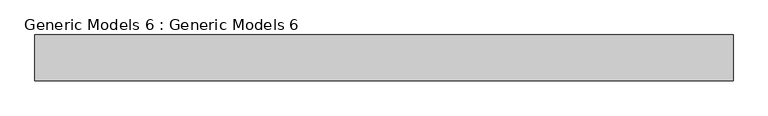
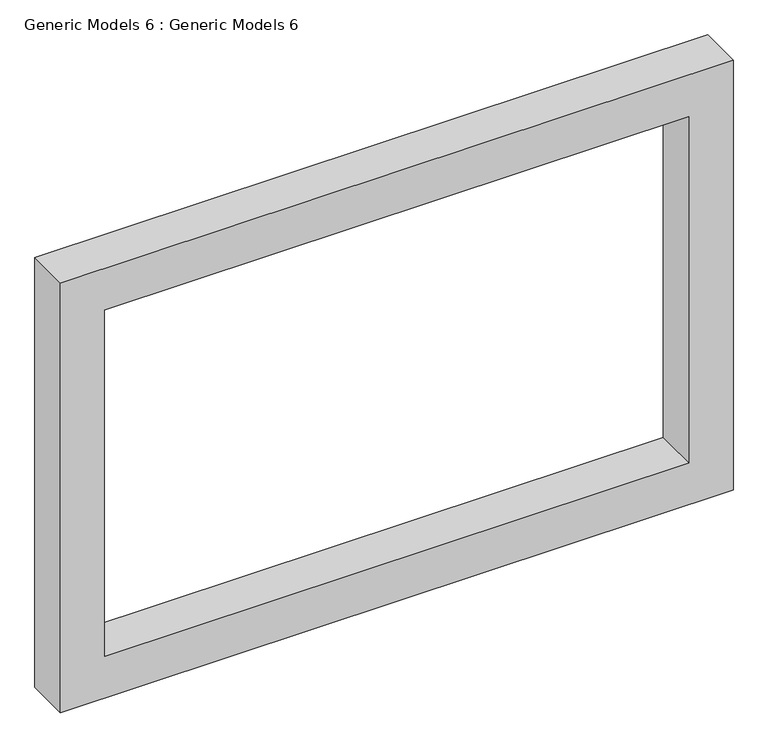
"""IFC4 building model written with IfcOpenShell, lengths in millimetres: proxy geometry, Generic Models 6 : Generic Models 6."""

from ifc_helpers import new_model, si_unit, frame, origin, place, context, project, spatial, polyline, outline, extrude, source, transform, mapped, element, save


def generic_models_6_generic_models_6_ad273a16(model_context):
    return source(origin(), model_context, "Body", "SweptSolid", [
        extrude(outline(polyline([(6070.0, -3351.3474631), (6070.0, -5666.1474631), (4505.2, -5666.1474631), (4505.2, -3351.3474631), (6070.0, -3351.3474631)]), holes=[polyline([(5917.6, -3503.7474631), (4657.6, -3503.7474631), (4657.6, -5513.7474631), (5917.6, -5513.7474631), (5917.6, -3503.7474631)])]), frame((0.0, -4424.6938352, 0.0), z_axis=(0.0, 1.0, 0.0), x_axis=(0.0, 0.0, 1.0)), (0.0, 0.0, 1.0), 152.4),
    ])


if __name__ == "__main__":
    model = new_model("IFC4")
    model_context = context("Model", 3, world=origin())
    ifc_project = project(units=[si_unit("LENGTHUNIT", "METRE", prefix="MILLI")], contexts=[model_context])
    site = spatial("IfcSite", under=ifc_project)
    building = spatial("IfcBuilding", under=site)
    placement = place(None, origin())
    generic_models_6_generic_models_6_shape = generic_models_6_generic_models_6_ad273a16(model_context)
    element("IfcBuildingElementProxy", 1, Name="Generic Models 6 : Generic Models 6", ObjectType="Generic Models 6 : Generic Models 6", at=placement, inside=building, context=model_context, shape_type="MappedRepresentation", body=[
        mapped(generic_models_6_generic_models_6_shape, transform((0.0, 0.0, 0.0), x_axis=(1.0, 0.0, 0.0), y_axis=(0.0, 1.0, 0.0), z_axis=(0.0, 0.0, 1.0))),
    ])
    save(model, "model.ifc")

# Revit data of these elements
# Element 1 (IfcBuildingElementProxy, "Generic Models 6 : Generic Models 6")
#   Materials on its faces: "WALL PAINT"
# Materials
#   "WALL PAINT": class "Generic", colour RGB 120 120 120, transparency 0, Cost = 0
